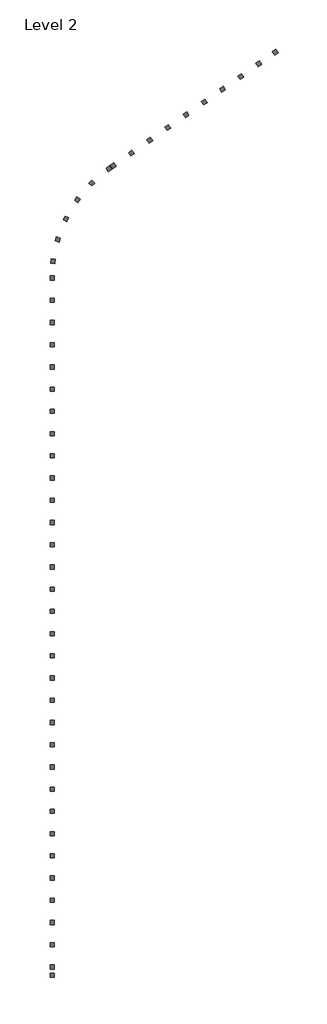
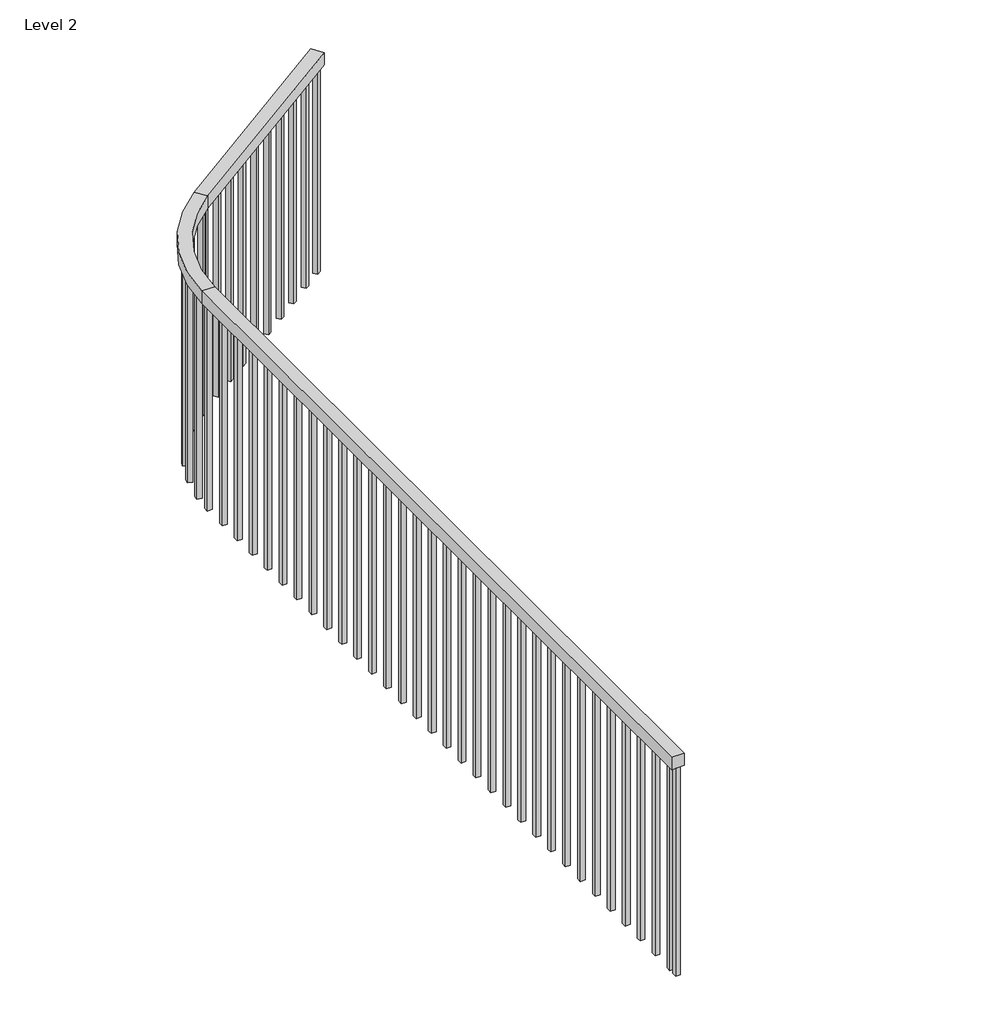
# One storey: 1 railing.
"""IFC4 building model written with IfcOpenShell, lengths in millimetres."""

from ifc_helpers import new_model, si_unit, frame, origin, place, context, project, spatial, polyline, circle_curve, outline, extrude, element, save
from ifc_brep_helpers import plane_surface, cylinder_surface, revolved_surface, advanced_brep

model = new_model("IFC4")

# Units and contexts
model_context = context("Model", 3, world=origin())
ifc_project = project(units=[si_unit("LENGTHUNIT", "METRE", prefix="MILLI")], contexts=[model_context])

# Site, building, storey
site = spatial("IfcSite", under=ifc_project)
building = spatial("IfcBuilding", under=site)
storey = spatial("IfcBuildingStorey", under=building, Name="Level 2", Elevation=3048.0)

# Railing
placement = place(None, origin())
element("IfcRailing", 1, ObjectType="Handrail - Rectangular", at=placement, inside=storey, context=model_context, shape_type="SolidModel", body=[
    advanced_brep(
    [(-15524.7542692, 2678.3932934, 4419.6), (-15524.7542692, 2678.3932934, 4368.8), (-15553.8919522, 2720.0062172, 4368.8), (-15553.8919522, 2720.0062172, 4419.6), (-16293.5064648, 2140.107211, 4419.6), (-16293.5064648, 2140.107211, 4368.8), (-16322.6441478, 2181.7201348, 4368.8), (-16322.6441478, 2181.7201348, 4419.6), (-16542.6231107, 1661.5585867, 4368.8), (-16542.6231107, 1661.5585867, 4419.6), (-16593.4231107, 1661.5585867, 4368.8), (-16593.4231107, 1661.5585867, 4419.6), (-16542.6231107, -1535.9534819, 4419.6), (-16593.4231107, -1535.9534819, 4419.6), (-16593.4231107, -1535.9534819, 4368.8), (-16542.6231107, -1535.9534819, 4368.8)],
    [
        (0, 1),
        (1, 2),
        (2, 3),
        (3, 0),
        (0, 4),
        (4, 5),
        (5, 1),
        (5, 6),
        (6, 2),
        (6, 7),
        (7, 3),
        (7, 4),
        (8, 5, circle_curve(frame((-15958.4231107, 1661.5585867, 4368.8), z_axis=(0.0, 0.0, -1.0), x_axis=(-0.5735764363510447, 0.8191520442889928, 0.0)), 584.2)),
        (4, 9, circle_curve(frame((-15958.4231107, 1661.5585867, 4419.6), z_axis=(0.0, 0.0, 1.0), x_axis=(-0.5735764363510447, 0.8191520442889928, 0.0)), 584.2)),
        (9, 8),
        (10, 6, circle_curve(frame((-15958.4231107, 1661.5585867, 4368.8), z_axis=(0.0, 0.0, -1.0), x_axis=(-0.5735764363510447, 0.8191520442889928, 0.0)), 635.0)),
        (8, 10),
        (11, 7, circle_curve(frame((-15958.4231107, 1661.5585867, 4419.6), z_axis=(0.0, 0.0, -1.0), x_axis=(-0.5735764363510447, 0.8191520442889928, 0.0)), 635.0)),
        (10, 11),
        (11, 9),
        (12, 13),
        (13, 14),
        (14, 15),
        (15, 12),
        (9, 12),
        (15, 8),
        (14, 10),
        (13, 11),
    ],
    [
        plane_surface(frame((-15539.3231107, 2699.1997553, 4419.6), z_axis=(0.8191520442889921, 0.5735764363510457, 0.0), x_axis=(0.5735764363510457, -0.8191520442889921, 0.0))),
        plane_surface(frame((-15524.7542692, 2678.3932934, 4419.6), z_axis=(0.5735764363510467, -0.8191520442889915, 0.0), x_axis=(-0.8191520442889915, -0.5735764363510467, 0.0))),
        plane_surface(frame((-15524.7542692, 2678.3932934, 4368.8), z_axis=(0.0, 0.0, -1.0000000000000002), x_axis=(-0.8191520442889915, -0.5735764363510467, 0.0))),
        plane_surface(frame((-15553.8919522, 2720.0062172, 4368.8), z_axis=(-0.5735764363510452, 0.8191520442889925, 0.0), x_axis=(-0.8191520442889925, -0.5735764363510452, 0.0))),
        plane_surface(frame((-15553.8919522, 2720.0062172, 4419.6), z_axis=(0.0, 0.0, 1.0), x_axis=(-0.8191520442889925, -0.5735764363510452, 0.0))),
        revolved_surface(polyline([(-16293.50646481628, 2140.1072109736297, 4419.6), (-16293.50646481628, 2140.1072109736297, 4368.8)]), (-15958.4231107, 1661.5585867, 4419.6), (0.0, 0.0, 1.0)),
        plane_surface(frame((-15958.4231107, 1661.5585867, 4368.8), z_axis=(0.0, 0.0, -1.0), x_axis=(-0.5735764363510447, 0.8191520442889928, 0.0))),
        cylinder_surface(frame((-15958.4231107, 1661.5585867, 4419.6), z_axis=(0.0, 0.0, 1.0), x_axis=(-0.5735764363510447, 0.8191520442889928, 0.0)), 635.0),
        plane_surface(frame((-15958.4231107, 1661.5585867, 4419.6), z_axis=(0.0, 0.0, 1.0), x_axis=(-0.5735764363510447, 0.8191520442889928, 0.0))),
        plane_surface(frame((-16568.0231107, -1535.9534819, 4419.6), z_axis=(0.0, -1.0, 0.0), x_axis=(0.0, 0.0, -1.0))),
        plane_surface(frame((-16542.6231107, 1661.5585867, 4419.6), z_axis=(1.0, 0.0, 0.0), x_axis=(0.0, -1.0, 0.0))),
        plane_surface(frame((-16542.6231107, 1661.5585867, 4368.8), z_axis=(0.0, 0.0, -1.0), x_axis=(0.0, -1.0, 0.0))),
        plane_surface(frame((-16593.4231107, 1661.5585867, 4368.8), z_axis=(-1.0, 0.0, 0.0), x_axis=(0.0, -1.0, 0.0))),
        plane_surface(frame((-16593.4231107, 1661.5585867, 4419.6), z_axis=(0.0, 0.0, 1.0), x_axis=(0.0, -1.0, 0.0))),
    ],
    [
        (0, [[1, 2, 3, 4]]),
        (1, [[-1, 5, 6, 7]]),
        (2, [[-2, -7, 8, 9]]),
        (3, [[-3, -9, 10, 11]]),
        (4, [[-4, -11, 12, -5]]),
        (5, [[13, -6, 14, 15]]),
        (6, [[16, -8, -13, 17]]),
        (7, [[18, -10, -16, 19]]),
        (8, [[-14, -12, -18, 20]]),
        (9, [[21, 22, 23, 24]]),
        (10, [[-15, 25, -24, 26]]),
        (11, [[-17, -26, -23, 27]]),
        (12, [[-19, -27, -22, 28]]),
        (13, [[-20, -28, -21, -25]]),
    ],
),
    extrude(outline(polyline([(-16577.5481107, -1478.5164133), (-16558.4981107, -1478.5164133), (-16558.4981107, -1497.5664133), (-16577.5481107, -1497.5664133), (-16577.5481107, -1478.5164133)])), frame((0.0, 0.0, 3505.2), z_axis=(0.0, 0.0, 1.0), x_axis=(1.0, 0.0, 0.0)), (0.0, 0.0, 1.0), 863.6),
    extrude(outline(polyline([(-16577.5481107, -1376.9164133), (-16558.4981107, -1376.9164133), (-16558.4981107, -1395.9664133), (-16577.5481107, -1395.9664133), (-16577.5481107, -1376.9164133)])), frame((0.0, 0.0, 3505.2), z_axis=(0.0, 0.0, 1.0), x_axis=(1.0, 0.0, 0.0)), (0.0, 0.0, 1.0), 863.6),
    extrude(outline(polyline([(-16577.5481107, -1275.3164133), (-16558.4981107, -1275.3164133), (-16558.4981107, -1294.3664133), (-16577.5481107, -1294.3664133), (-16577.5481107, -1275.3164133)])), frame((0.0, 0.0, 3505.2), z_axis=(0.0, 0.0, 1.0), x_axis=(1.0, 0.0, 0.0)), (0.0, 0.0, 1.0), 863.6),
    extrude(outline(polyline([(-16577.5481107, -1173.7164133), (-16558.4981107, -1173.7164133), (-16558.4981107, -1192.7664133), (-16577.5481107, -1192.7664133), (-16577.5481107, -1173.7164133)])), frame((0.0, 0.0, 3505.2), z_axis=(0.0, 0.0, 1.0), x_axis=(1.0, 0.0, 0.0)), (0.0, 0.0, 1.0), 863.6),
    extrude(outline(polyline([(-16577.5481107, -1072.1164133), (-16558.4981107, -1072.1164133), (-16558.4981107, -1091.1664133), (-16577.5481107, -1091.1664133), (-16577.5481107, -1072.1164133)])), frame((0.0, 0.0, 3505.2), z_axis=(0.0, 0.0, 1.0), x_axis=(1.0, 0.0, 0.0)), (0.0, 0.0, 1.0), 863.6),
    extrude(outline(polyline([(-16577.5481107, -970.5164133), (-16558.4981107, -970.5164133), (-16558.4981107, -989.5664133), (-16577.5481107, -989.5664133), (-16577.5481107, -970.5164133)])), frame((0.0, 0.0, 3505.2), z_axis=(0.0, 0.0, 1.0), x_axis=(1.0, 0.0, 0.0)), (0.0, 0.0, 1.0), 863.6),
    extrude(outline(polyline([(-16577.5481107, -868.9164133), (-16558.4981107, -868.9164133), (-16558.4981107, -887.9664133), (-16577.5481107, -887.9664133), (-16577.5481107, -868.9164133)])), frame((0.0, 0.0, 3505.2), z_axis=(0.0, 0.0, 1.0), x_axis=(1.0, 0.0, 0.0)), (0.0, 0.0, 1.0), 863.6),
    extrude(outline(polyline([(-16577.5481107, -767.3164133), (-16558.4981107, -767.3164133), (-16558.4981107, -786.3664133), (-16577.5481107, -786.3664133), (-16577.5481107, -767.3164133)])), frame((0.0, 0.0, 3505.2), z_axis=(0.0, 0.0, 1.0), x_axis=(1.0, 0.0, 0.0)), (0.0, 0.0, 1.0), 863.6),
    extrude(outline(polyline([(-16577.5481107, -665.7164133), (-16558.4981107, -665.7164133), (-16558.4981107, -684.7664133), (-16577.5481107, -684.7664133), (-16577.5481107, -665.7164133)])), frame((0.0, 0.0, 3505.2), z_axis=(0.0, 0.0, 1.0), x_axis=(1.0, 0.0, 0.0)), (0.0, 0.0, 1.0), 863.6),
    extrude(outline(polyline([(-16577.5481107, -564.1164133), (-16558.4981107, -564.1164133), (-16558.4981107, -583.1664133), (-16577.5481107, -583.1664133), (-16577.5481107, -564.1164133)])), frame((0.0, 0.0, 3505.2), z_axis=(0.0, 0.0, 1.0), x_axis=(1.0, 0.0, 0.0)), (0.0, 0.0, 1.0), 863.6),
    extrude(outline(polyline([(-16577.5481107, -462.5164133), (-16558.4981107, -462.5164133), (-16558.4981107, -481.5664133), (-16577.5481107, -481.5664133), (-16577.5481107, -462.5164133)])), frame((0.0, 0.0, 3505.2), z_axis=(0.0, 0.0, 1.0), x_axis=(1.0, 0.0, 0.0)), (0.0, 0.0, 1.0), 863.6),
    extrude(outline(polyline([(-16577.5481107, -360.9164133), (-16558.4981107, -360.9164133), (-16558.4981107, -379.9664133), (-16577.5481107, -379.9664133), (-16577.5481107, -360.9164133)])), frame((0.0, 0.0, 3505.2), z_axis=(0.0, 0.0, 1.0), x_axis=(1.0, 0.0, 0.0)), (0.0, 0.0, 1.0), 863.6),
    extrude(outline(polyline([(-16577.5481107, -259.3164133), (-16558.4981107, -259.3164133), (-16558.4981107, -278.3664133), (-16577.5481107, -278.3664133), (-16577.5481107, -259.3164133)])), frame((0.0, 0.0, 3505.2), z_axis=(0.0, 0.0, 1.0), x_axis=(1.0, 0.0, 0.0)), (0.0, 0.0, 1.0), 863.6),
    extrude(outline(polyline([(-16577.5481107, -157.7164133), (-16558.4981107, -157.7164133), (-16558.4981107, -176.7664133), (-16577.5481107, -176.7664133), (-16577.5481107, -157.7164133)])), frame((0.0, 0.0, 3505.2), z_axis=(0.0, 0.0, 1.0), x_axis=(1.0, 0.0, 0.0)), (0.0, 0.0, 1.0), 863.6),
    extrude(outline(polyline([(-16577.5481107, -56.1164133), (-16558.4981107, -56.1164133), (-16558.4981107, -75.1664133), (-16577.5481107, -75.1664133), (-16577.5481107, -56.1164133)])), frame((0.0, 0.0, 3505.2), z_axis=(0.0, 0.0, 1.0), x_axis=(1.0, 0.0, 0.0)), (0.0, 0.0, 1.0), 863.6),
    extrude(outline(polyline([(-16577.5481107, 45.4835867), (-16558.4981107, 45.4835867), (-16558.4981107, 26.4335867), (-16577.5481107, 26.4335867), (-16577.5481107, 45.4835867)])), frame((0.0, 0.0, 3505.2), z_axis=(0.0, 0.0, 1.0), x_axis=(1.0, 0.0, 0.0)), (0.0, 0.0, 1.0), 863.6),
    extrude(outline(polyline([(-16577.5481107, 147.0835867), (-16558.4981107, 147.0835867), (-16558.4981107, 128.0335867), (-16577.5481107, 128.0335867), (-16577.5481107, 147.0835867)])), frame((0.0, 0.0, 3505.2), z_axis=(0.0, 0.0, 1.0), x_axis=(1.0, 0.0, 0.0)), (0.0, 0.0, 1.0), 863.6),
    extrude(outline(polyline([(-16577.5481107, 248.6835867), (-16558.4981107, 248.6835867), (-16558.4981107, 229.6335867), (-16577.5481107, 229.6335867), (-16577.5481107, 248.6835867)])), frame((0.0, 0.0, 3505.2), z_axis=(0.0, 0.0, 1.0), x_axis=(1.0, 0.0, 0.0)), (0.0, 0.0, 1.0), 863.6),
    extrude(outline(polyline([(-16577.5481107, 350.2835867), (-16558.4981107, 350.2835867), (-16558.4981107, 331.2335867), (-16577.5481107, 331.2335867), (-16577.5481107, 350.2835867)])), frame((0.0, 0.0, 3505.2), z_axis=(0.0, 0.0, 1.0), x_axis=(1.0, 0.0, 0.0)), (0.0, 0.0, 1.0), 863.6),
    extrude(outline(polyline([(-16577.5481107, 451.8835867), (-16558.4981107, 451.8835867), (-16558.4981107, 432.8335867), (-16577.5481107, 432.8335867), (-16577.5481107, 451.8835867)])), frame((0.0, 0.0, 3505.2), z_axis=(0.0, 0.0, 1.0), x_axis=(1.0, 0.0, 0.0)), (0.0, 0.0, 1.0), 863.6),
    extrude(outline(polyline([(-16577.5481107, 553.4835867), (-16558.4981107, 553.4835867), (-16558.4981107, 534.4335867), (-16577.5481107, 534.4335867), (-16577.5481107, 553.4835867)])), frame((0.0, 0.0, 3505.2), z_axis=(0.0, 0.0, 1.0), x_axis=(1.0, 0.0, 0.0)), (0.0, 0.0, 1.0), 863.6),
    extrude(outline(polyline([(-16577.5481107, 655.0835867), (-16558.4981107, 655.0835867), (-16558.4981107, 636.0335867), (-16577.5481107, 636.0335867), (-16577.5481107, 655.0835867)])), frame((0.0, 0.0, 3505.2), z_axis=(0.0, 0.0, 1.0), x_axis=(1.0, 0.0, 0.0)), (0.0, 0.0, 1.0), 863.6),
    extrude(outline(polyline([(-16577.5481107, 756.6835867), (-16558.4981107, 756.6835867), (-16558.4981107, 737.6335867), (-16577.5481107, 737.6335867), (-16577.5481107, 756.6835867)])), frame((0.0, 0.0, 3505.2), z_axis=(0.0, 0.0, 1.0), x_axis=(1.0, 0.0, 0.0)), (0.0, 0.0, 1.0), 863.6),
    extrude(outline(polyline([(-16577.5481107, 858.2835867), (-16558.4981107, 858.2835867), (-16558.4981107, 839.2335867), (-16577.5481107, 839.2335867), (-16577.5481107, 858.2835867)])), frame((0.0, 0.0, 3505.2), z_axis=(0.0, 0.0, 1.0), x_axis=(1.0, 0.0, 0.0)), (0.0, 0.0, 1.0), 863.6),
    extrude(outline(polyline([(-16577.5481107, 959.8835867), (-16558.4981107, 959.8835867), (-16558.4981107, 940.8335867), (-16577.5481107, 940.8335867), (-16577.5481107, 959.8835867)])), frame((0.0, 0.0, 3505.2), z_axis=(0.0, 0.0, 1.0), x_axis=(1.0, 0.0, 0.0)), (0.0, 0.0, 1.0), 863.6),
    extrude(outline(polyline([(-16577.5481107, 1061.4835867), (-16558.4981107, 1061.4835867), (-16558.4981107, 1042.4335867), (-16577.5481107, 1042.4335867), (-16577.5481107, 1061.4835867)])), frame((0.0, 0.0, 3505.2), z_axis=(0.0, 0.0, 1.0), x_axis=(1.0, 0.0, 0.0)), (0.0, 0.0, 1.0), 863.6),
    extrude(outline(polyline([(-16577.5481107, 1163.0835867), (-16558.4981107, 1163.0835867), (-16558.4981107, 1144.0335867), (-16577.5481107, 1144.0335867), (-16577.5481107, 1163.0835867)])), frame((0.0, 0.0, 3505.2), z_axis=(0.0, 0.0, 1.0), x_axis=(1.0, 0.0, 0.0)), (0.0, 0.0, 1.0), 863.6),
    extrude(outline(polyline([(-16577.5481107, 1264.6835867), (-16558.4981107, 1264.6835867), (-16558.4981107, 1245.6335867), (-16577.5481107, 1245.6335867), (-16577.5481107, 1264.6835867)])), frame((0.0, 0.0, 3505.2), z_axis=(0.0, 0.0, 1.0), x_axis=(1.0, 0.0, 0.0)), (0.0, 0.0, 1.0), 863.6),
    extrude(outline(polyline([(-16577.5481107, 1366.2835867), (-16558.4981107, 1366.2835867), (-16558.4981107, 1347.2335867), (-16577.5481107, 1347.2335867), (-16577.5481107, 1366.2835867)])), frame((0.0, 0.0, 3505.2), z_axis=(0.0, 0.0, 1.0), x_axis=(1.0, 0.0, 0.0)), (0.0, 0.0, 1.0), 863.6),
    extrude(outline(polyline([(-16577.5481107, 1467.8835867), (-16558.4981107, 1467.8835867), (-16558.4981107, 1448.8335867), (-16577.5481107, 1448.8335867), (-16577.5481107, 1467.8835867)])), frame((0.0, 0.0, 3505.2), z_axis=(0.0, 0.0, 1.0), x_axis=(1.0, 0.0, 0.0)), (0.0, 0.0, 1.0), 863.6),
    extrude(outline(polyline([(-16577.5481107, 1569.4835867), (-16558.4981107, 1569.4835867), (-16558.4981107, 1550.4335867), (-16577.5481107, 1550.4335867), (-16577.5481107, 1569.4835867)])), frame((0.0, 0.0, 3505.2), z_axis=(0.0, 0.0, 1.0), x_axis=(1.0, 0.0, 0.0)), (0.0, 0.0, 1.0), 863.6),
    extrude(outline(polyline([(-16571.3907526, 1749.1779975), (-16552.493206, 1746.7727471), (-16554.8984563, 1727.8752004), (-16573.796003, 1730.2804508), (-16571.3907526, 1749.1779975)])), frame((0.0, 0.0, 3505.2), z_axis=(0.0, 0.0, 1.0), x_axis=(1.0, 0.0, 0.0)), (0.0, 0.0, 1.0), 863.6),
    extrude(outline(polyline([(-16548.3612806, 1849.6528369), (-16530.1246146, 1844.1458856), (-16535.6315658, 1825.9092196), (-16553.8682319, 1831.4161709), (-16548.3612806, 1849.6528369)])), frame((0.0, 0.0, 3505.2), z_axis=(0.0, 0.0, 1.0), x_axis=(1.0, 0.0, 0.0)), (0.0, 0.0, 1.0), 863.6),
    extrude(outline(polyline([(-16508.9825353, 1944.9149193), (-16491.9121524, 1936.4588842), (-16500.3681876, 1919.3885014), (-16517.4385704, 1927.8445365), (-16508.9825353, 1944.9149193)])), frame((0.0, 0.0, 3505.2), z_axis=(0.0, 0.0, 1.0), x_axis=(1.0, 0.0, 0.0)), (0.0, 0.0, 1.0), 863.6),
    extrude(outline(polyline([(-16454.3458411, 2032.3241956), (-16438.9148221, 2021.1534233), (-16450.0855944, 2005.7224043), (-16465.5166133, 2016.8931766), (-16454.3458411, 2032.3241956)])), frame((0.0, 0.0, 3505.2), z_axis=(0.0, 0.0, 1.0), x_axis=(1.0, 0.0, 0.0)), (0.0, 0.0, 1.0), 863.6),
    extrude(outline(polyline([(-16385.965374, 2109.4582455), (-16372.601367, 2095.8823177), (-16386.1772948, 2082.5183107), (-16399.5413018, 2096.0942385), (-16385.965374, 2109.4582455)])), frame((0.0, 0.0, 3505.2), z_axis=(0.0, 0.0, 1.0), x_axis=(1.0, 0.0, 0.0)), (0.0, 0.0, 1.0), 863.6),
    extrude(outline(polyline([(-16286.0166323, 2187.9872007), (-16275.0900012, 2172.3823542), (-16290.6948476, 2161.4557231), (-16301.6214787, 2177.0605696), (-16286.0166323, 2187.9872007)])), frame((0.0, 0.0, 3505.2), z_axis=(0.0, 0.0, 1.0), x_axis=(1.0, 0.0, 0.0)), (0.0, 0.0, 1.0), 863.6),
    extrude(outline(polyline([(-16202.7907846, 2246.2625666), (-16191.8641535, 2230.6577202), (-16207.4689999, 2219.7310891), (-16218.395631, 2235.3359355), (-16202.7907846, 2246.2625666)])), frame((0.0, 0.0, 3505.2), z_axis=(0.0, 0.0, 1.0), x_axis=(1.0, 0.0, 0.0)), (0.0, 0.0, 1.0), 863.6),
    extrude(outline(polyline([(-16119.5649369, 2304.5379325), (-16108.6383058, 2288.9330861), (-16124.2431522, 2278.006455), (-16135.1697833, 2293.6113014), (-16119.5649369, 2304.5379325)])), frame((0.0, 0.0, 3505.2), z_axis=(0.0, 0.0, 1.0), x_axis=(1.0, 0.0, 0.0)), (0.0, 0.0, 1.0), 863.6),
    extrude(outline(polyline([(-16036.3390892, 2362.8132985), (-16025.4124581, 2347.208452), (-16041.0173045, 2336.2818209), (-16051.9439356, 2351.8866674), (-16036.3390892, 2362.8132985)])), frame((0.0, 0.0, 3505.2), z_axis=(0.0, 0.0, 1.0), x_axis=(1.0, 0.0, 0.0)), (0.0, 0.0, 1.0), 863.6),
    extrude(outline(polyline([(-15953.1132415, 2421.0886644), (-15942.1866104, 2405.483818), (-15957.7914568, 2394.5571869), (-15968.7180879, 2410.1620333), (-15953.1132415, 2421.0886644)])), frame((0.0, 0.0, 3505.2), z_axis=(0.0, 0.0, 1.0), x_axis=(1.0, 0.0, 0.0)), (0.0, 0.0, 1.0), 863.6),
    extrude(outline(polyline([(-15869.8873938, 2479.3640303), (-15858.9607627, 2463.7591839), (-15874.5656091, 2452.8325528), (-15885.4922402, 2468.4373992), (-15869.8873938, 2479.3640303)])), frame((0.0, 0.0, 3505.2), z_axis=(0.0, 0.0, 1.0), x_axis=(1.0, 0.0, 0.0)), (0.0, 0.0, 1.0), 863.6),
    extrude(outline(polyline([(-15786.6615461, 2537.6393963), (-15775.734915, 2522.0345498), (-15791.3397614, 2511.1079187), (-15802.2663925, 2526.7127652), (-15786.6615461, 2537.6393963)])), frame((0.0, 0.0, 3505.2), z_axis=(0.0, 0.0, 1.0), x_axis=(1.0, 0.0, 0.0)), (0.0, 0.0, 1.0), 863.6),
    extrude(outline(polyline([(-15703.4356984, 2595.9147622), (-15692.5090673, 2580.3099158), (-15708.1139137, 2569.3832847), (-15719.0405448, 2584.9881311), (-15703.4356984, 2595.9147622)])), frame((0.0, 0.0, 3505.2), z_axis=(0.0, 0.0, 1.0), x_axis=(1.0, 0.0, 0.0)), (0.0, 0.0, 1.0), 863.6),
    extrude(outline(polyline([(-15620.2098507, 2654.1901281), (-15609.2832196, 2638.5852817), (-15624.888066, 2627.6586506), (-15635.8146971, 2643.263497), (-15620.2098507, 2654.1901281)])), frame((0.0, 0.0, 3505.2), z_axis=(0.0, 0.0, 1.0), x_axis=(1.0, 0.0, 0.0)), (0.0, 0.0, 1.0), 863.6),
    extrude(outline(polyline([(-16577.5481107, 1671.0835867), (-16558.4981107, 1671.0835867), (-16558.4981107, 1652.0335867), (-16577.5481107, 1652.0335867), (-16577.5481107, 1671.0835867)])), frame((0.0, 0.0, 3505.2), z_axis=(0.0, 0.0, 1.0), x_axis=(1.0, 0.0, 0.0)), (0.0, 0.0, 1.0), 863.6),
    extrude(outline(polyline([(-16305.7361986, 2174.1794117), (-16294.8095675, 2158.5745653), (-16310.4144139, 2147.6479341), (-16321.341045, 2163.2527806), (-16305.7361986, 2174.1794117)])), frame((0.0, 0.0, 3505.2), z_axis=(0.0, 0.0, 1.0), x_axis=(1.0, 0.0, 0.0)), (0.0, 0.0, 1.0), 863.6),
    extrude(outline(polyline([(-16577.5481107, -1516.9034819), (-16558.4981107, -1516.9034819), (-16558.4981107, -1535.9534819), (-16577.5481107, -1535.9534819), (-16577.5481107, -1516.9034819)])), frame((0.0, 0.0, 3505.2), z_axis=(0.0, 0.0, 1.0), x_axis=(1.0, 0.0, 0.0)), (0.0, 0.0, 1.0), 863.6),
    extrude(outline(polyline([(-15544.7864262, 2707.0021785), (-15533.8597951, 2691.3973321), (-15549.4646416, 2680.470701), (-15560.3912727, 2696.0755474), (-15544.7864262, 2707.0021785)])), frame((0.0, 0.0, 3505.2), z_axis=(0.0, 0.0, 1.0), x_axis=(1.0, 0.0, 0.0)), (0.0, 0.0, 1.0), 863.6),
])

save(model, "model.ifc")

# Revit data of these elements
# Type "Handrail - Rectangular"
#   Assembly Code = "C2010400"
#   built-in parameter 1008612 = 0.0416667 (stored number, unit not read)
#   built-in parameter 1008611 = 0.0416667 (stored number, unit not read)
#   built-in parameter 1008609 = 0.333333 (stored number, unit not read)
#   built-in parameter 1008604 = 0.166667 (stored number, unit not read)
#   built-in parameter 1008603 = 0.166667 (stored number, unit not read)
#   Railing Height = 3' - 0"
#   built-in parameter 1008630 = 2
#   built-in parameter 1008610 = 2
#   built-in parameter 1008618 = Baluster - Square : 3/4"
# Element 1 (IfcRailing, "Handrail - Rectangular")
#   built-in parameter 1008621 = 1.5 (stored number, unit not read)
#   Phase Created = New Construction
